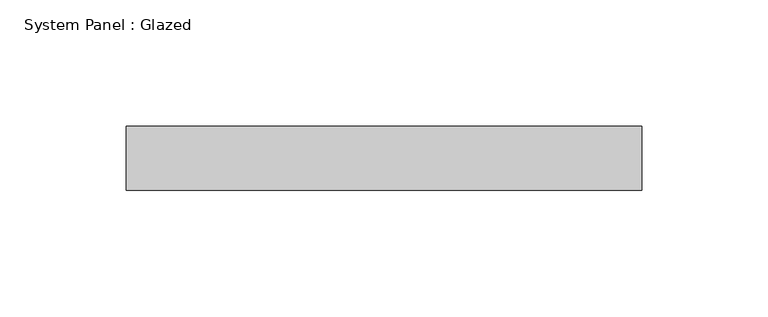
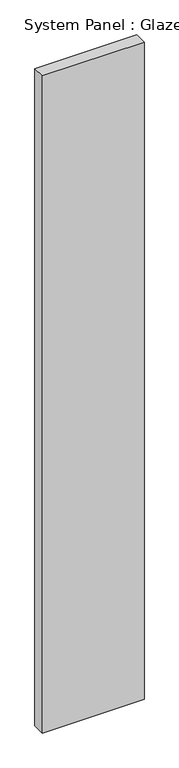
"""IFC4 building model written with IfcOpenShell, lengths in millimetres: plate geometry, System Panel : Glazed."""

from ifc_helpers import new_model, si_unit, origin, origin_with_axes, place, context, project, spatial, polyline, outline, extrude, source, transform, mapped, element, save


def system_panel_glazed_d23cfa45(model_context):
    return source(origin(), model_context, "Body", "SweptSolid", [
        extrude(outline(polyline([(102.235, 19.05), (-102.235, 19.05), (-102.235, 44.45), (102.235, 44.45), (102.235, 19.05)])), origin_with_axes(), (0.0, 0.0, 1.0), 1395.1131867),
    ])


if __name__ == "__main__":
    model = new_model("IFC4")
    model_context = context("Model", 3, world=origin())
    ifc_project = project(units=[si_unit("LENGTHUNIT", "METRE", prefix="MILLI")], contexts=[model_context])
    site = spatial("IfcSite", under=ifc_project)
    building = spatial("IfcBuilding", under=site)
    placement = place(None, origin())
    system_panel_glazed_shape = system_panel_glazed_d23cfa45(model_context)
    element("IfcPlate", 1, ObjectType="System Panel : Glazed", at=placement, inside=building, context=model_context, shape_type="MappedRepresentation", body=[
        mapped(system_panel_glazed_shape, transform((0.0, 0.0, 0.0), x_axis=(1.0, 0.0, 0.0), y_axis=(0.0, 1.0, 0.0), z_axis=(0.0, 0.0, 1.0))),
    ])
    save(model, "model.ifc")

# Revit data of these elements
# Type "System Panel : Glazed"
#   Construction Type Id = "GSP4R"
#   Analytic Construction = "1/8 in Pilkington single glazing"
#   Visual Light Transmittance = 0.9
#   Solar Heat Gain Coefficient = 0.86
#   Heat Transfer Coefficient (U) = 1.18115 BTU/(h·ft²·°F)
#   Define Thermal Properties by = 1
# Element 1 (IfcPlate, "System Panel : Glazed")
#   Materials on its faces: "Glass"
# Materials
#   "Glass": class "Glass", colour RGB 0 128 192, transparency 0.75, Description = "Soda Lime Glass", Cost = 0
